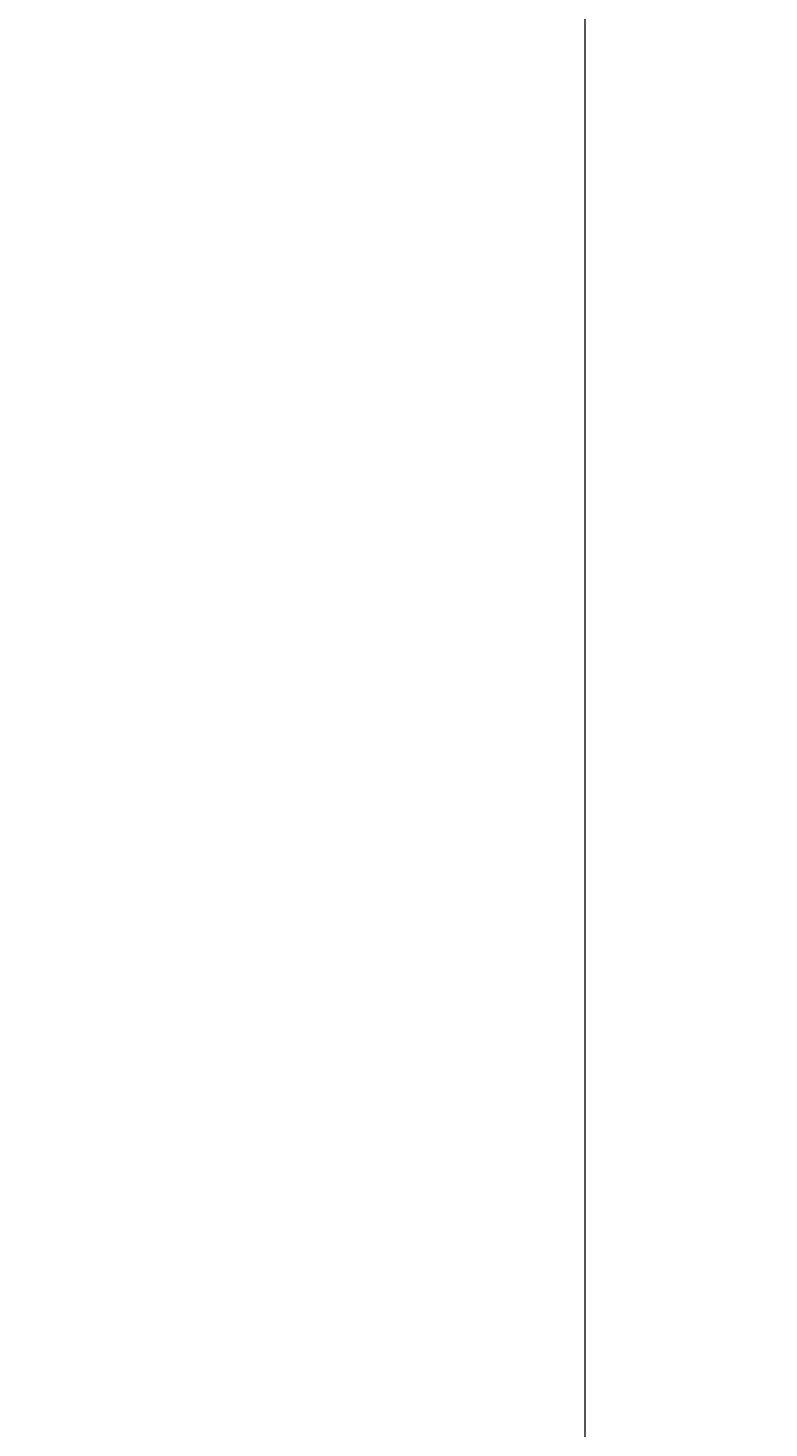
# Model space of a CAD drawing. Units: inches. Extents: x 1885 to 2748, y 783 to 2421.
# Tile 77 of 117: x 2004 to 2017, y 2120 to 2144. Entities that reach past the tile are written whole.
import ezdxf

# ---------------------------------------------------------------- set-up
doc = ezdxf.new("R2010")
doc.units = ezdxf.units.IN
doc.layers.add('A-ANNO-DIMS', color=2, linetype='Continuous', lineweight=18)
doc.layers.add('A-FLOR-CASE', color=9, linetype='Continuous', lineweight=18)
doc.styles.get("Standard").update_dxf_attribs({"font": 'arial.ttf'})
doc.dimstyles.get("Standard").update_dxf_attribs({"dimtxt": 0.18, "dimasz": 0.18, "dimexe": 0.18, "dimexo": 0.0625, "dimgap": 0.09, "dimtad": 0, "dimtih": 1, "dimtoh": 1, "dimdec": 4, "dimzin": 0, "dimdsep": 46, "dimtxsty": 'Standard', "dimcen": 0.09, "dimadec": 0, "dimazin": 0, "dimtfac": 1, "dimtdec": 4, "dimtofl": 0, "dimtmove": 0, "dimatfit": 3, "dimfxl": 1, "dimtolj": 1, "dimtzin": 0, "dimarcsym": 0})

# ---------------------------------------------------------------- blocks, each defined once
blk = doc.blocks.new('*D48')
at = {"layer": 'A-ANNO-DIMS', "color": 0, "lineweight": -2, "transparency": 16777216}
for p, q in [((1980.711, 2348.006), (1902.844, 2348.006)), ((1903.024, 2347.826), (1903.024, 2114.937)), ((1903.024, 1881.686), (1903.024, 2114.574)), ((2016.711, 1881.506), (1902.844, 1881.506))]:
    blk.add_line(p, q, dxfattribs=at)
at = {"layer": 'A-ANNO-DIMS', "color": 0, "transparency": 16777216}
for points in [[(1902.994, 2347.826), (1903.054, 2347.826), (1903.024, 2348.006)], [(1902.994, 1881.686), (1903.054, 1881.686), (1903.024, 1881.506)]]:
    blk.add_solid(points, dxfattribs=at)
at = {"layer": 'Defpoints', "color": 0, "transparency": 16777216}
for p in [(1903.024, 2348.006), (1980.774, 2348.006), (2016.774, 1881.506)]:
    blk.add_point(p, dxfattribs=at)
at = {"layer": 'A-ANNO-DIMS', "color": 0, "transparency": 16777216, "insert": (1903.024, 2114.756), "char_height": 0.18, "attachment_point": 5}
blk.add_mtext('\\A1;466.5', dxfattribs=at)

msp = doc.modelspace()

# ---------------------------------------------------------------- linework, layer by layer
at = {"layer": 'A-FLOR-CASE'}
msp.add_line((2013.676, 2165.006), (2013.676, 2093.221), dxfattribs=at)

# ---------------------------------------------------------------- dimensions: what is measured, and where the dimension line sits
at = {"layer": 'A-ANNO-DIMS'}
dim = msp.add_linear_dim(base=(1903.024, 2348.006), p1=(2016.774, 1881.506), p2=(1980.774, 2348.006), angle=90, dimstyle='Standard', override={"dimdec": 1, "dimlfac": 1, "dimrnd": 0, "dimzin": 0, "dimdsep": 46, "dimlunit": 2}, dxfattribs=at)
dim.commit()
dim.dimension.update_dxf_attribs({"geometry": '*D48', "text_midpoint": (1903.024, 2114.756)})

doc.saveas('drawing.dxf')
